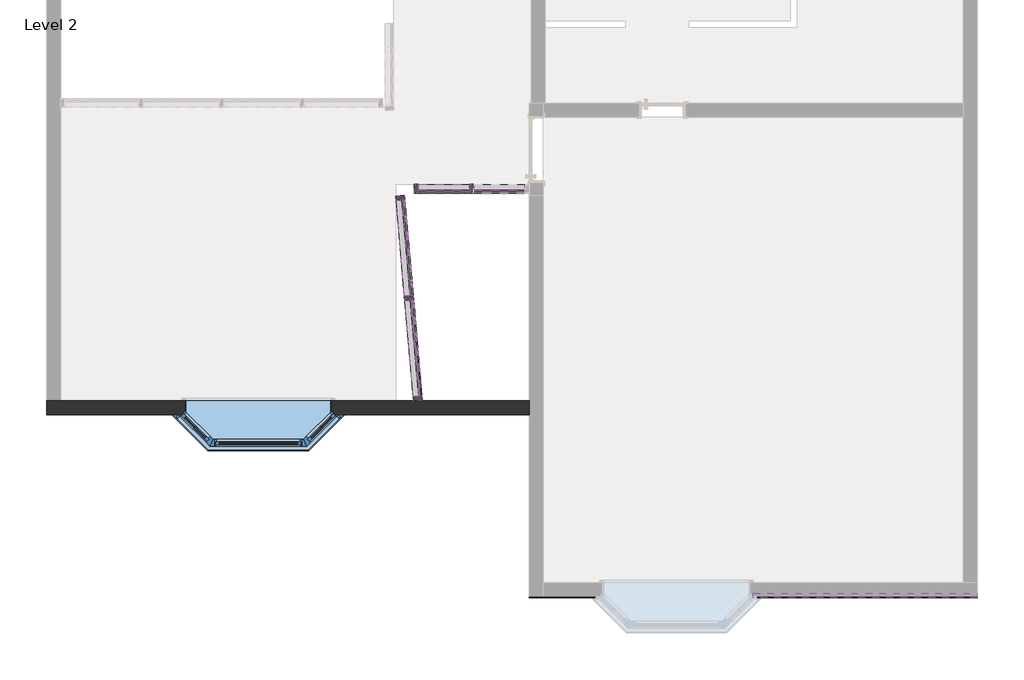
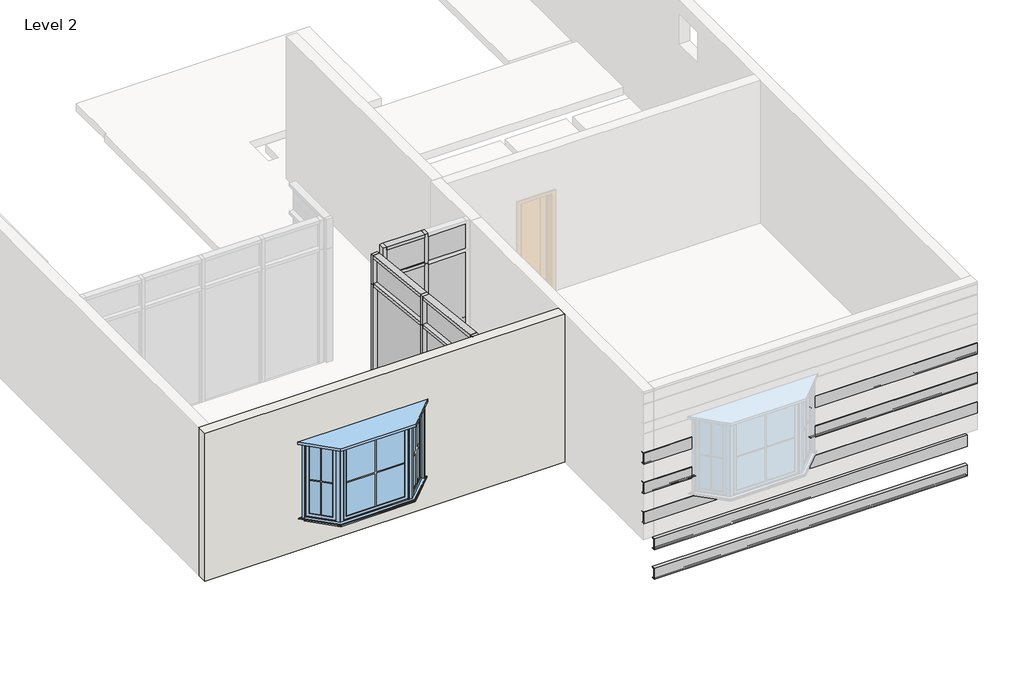
# One storey, part 2 of 5: 20 members, 8 plates, 5 proxies, 1 wall, 1 window.
"""IFC4 building model written with IfcOpenShell, lengths in millimetres."""

from ifc_helpers import new_model, si_unit, point, frame, frame_2d, origin, place, context, project, spatial, polyline, circle_curve, trimmed, segment, composite_curve, outline, extrude, faceted_brep, transform, mapped, element, save
from components import member_6e77e263, member_47bfaf8a, member_f0fea5a5, member_ee409385, member_3a0a7659, member_7b995701, member_d08ad361, member_d72f1a08, system_panel_glazed_0d615b27, system_panel_glazed_15008f27, system_panel_glazed_7a129d22, system_panel_glazed_9470322e, window_9f89e8e4

model = new_model("IFC4")

# Units and contexts
model_context = context("Model", 3, world=origin())
ifc_project = project(units=[si_unit("LENGTHUNIT", "METRE", prefix="MILLI")], contexts=[model_context])

# Site, building, storey
site = spatial("IfcSite", under=ifc_project)
building = spatial("IfcBuilding", under=site)
storey = spatial("IfcBuildingStorey", under=building, Name="Level 2", Elevation=3048.0)

# Proxies
placement = place(None, origin())
element("IfcBuildingElementProxy", 1, Name="Reveal", ObjectType="Reveal", at=placement, inside=storey, context=model_context, shape_type="SweptSolid", body=[
    extrude(outline(composite_curve([segment(polyline([(-10015.9757973, 3619.5), (-9952.7297973, 3619.5), (-9952.7297973, 3618.1203242)]), True, "CONTINUOUS"), segment(trimmed(circle_curve(frame_2d((-9957.9748973, 3618.1203242)), 5.2451), [point((-9952.7297973, 3618.1203242))], [point((-9957.1126065, 3612.9465897))], False, "CARTESIAN"), True, "CONTINUOUS"), segment(polyline([(-9957.1126065, 3612.9465897), (-9980.7332973, 3609.0098), (-9999.9711789, 3605.80348)]), True, "CONTINUOUS"), segment(trimmed(circle_curve(frame_2d((-9998.2465973, 3595.456011)), 10.4902), [point((-9999.9711789, 3605.80348))], [point((-10008.7367973, 3595.456011))], True, "CARTESIAN"), True, "CONTINUOUS"), segment(polyline([(-10008.7367973, 3595.456011), (-10008.7367973, 3414.943989)]), True, "CONTINUOUS"), segment(trimmed(circle_curve(frame_2d((-9998.2465973, 3414.943989)), 10.4902), [point((-10008.7367973, 3414.943989))], [point((-9999.9711789, 3404.59652))], True, "CARTESIAN"), True, "CONTINUOUS"), segment(polyline([(-9999.9711789, 3404.59652), (-9980.7332973, 3401.3902), (-9957.1126065, 3397.4534103)]), True, "CONTINUOUS"), segment(trimmed(circle_curve(frame_2d((-9957.9748973, 3392.2796758)), 5.2451), [point((-9957.1126065, 3397.4534103))], [point((-9952.7297973, 3392.2796758))], False, "CARTESIAN"), True, "CONTINUOUS"), segment(polyline([(-9952.7297973, 3392.2796758), (-9952.7297973, 3390.9), (-10015.9757973, 3390.9), (-10015.9757973, 3619.5)]), True, "CONTINUOUS")], self_intersect=False)), frame((-43748.9380314, 0.0, 0.0), z_axis=(1.0, 0.0, 0.0), x_axis=(0.0, 1.0, 0.0)), (0.0, 0.0, 1.0), 6502.4),
])
element("IfcBuildingElementProxy", 2, Name="Reveal", ObjectType="Reveal", at=placement, inside=storey, context=model_context, shape_type="SweptSolid", body=[
    extrude(outline(composite_curve([segment(polyline([(-10015.9757973, 4229.1), (-9952.7297973, 4229.1), (-9952.7297973, 4227.7203242)]), True, "CONTINUOUS"), segment(trimmed(circle_curve(frame_2d((-9957.9748973, 4227.7203242)), 5.2451), [point((-9952.7297973, 4227.7203242))], [point((-9957.1126065, 4222.5465897))], False, "CARTESIAN"), True, "CONTINUOUS"), segment(polyline([(-9957.1126065, 4222.5465897), (-9980.7332973, 4218.6098), (-9999.9711789, 4215.40348)]), True, "CONTINUOUS"), segment(trimmed(circle_curve(frame_2d((-9998.2465973, 4205.056011)), 10.4902), [point((-9999.9711789, 4215.40348))], [point((-10008.7367973, 4205.056011))], True, "CARTESIAN"), True, "CONTINUOUS"), segment(polyline([(-10008.7367973, 4205.056011), (-10008.7367973, 4024.543989)]), True, "CONTINUOUS"), segment(trimmed(circle_curve(frame_2d((-9998.2465973, 4024.543989)), 10.4902), [point((-10008.7367973, 4024.543989))], [point((-9999.9711789, 4014.19652))], True, "CARTESIAN"), True, "CONTINUOUS"), segment(polyline([(-9999.9711789, 4014.19652), (-9980.7332973, 4010.9902), (-9957.1126065, 4007.0534103)]), True, "CONTINUOUS"), segment(trimmed(circle_curve(frame_2d((-9957.9748973, 4001.8796758)), 5.2451), [point((-9957.1126065, 4007.0534103))], [point((-9952.7297973, 4001.8796758))], False, "CARTESIAN"), True, "CONTINUOUS"), segment(polyline([(-9952.7297973, 4001.8796758), (-9952.7297973, 4000.5), (-10015.9757973, 4000.5), (-10015.9757973, 4229.1)]), True, "CONTINUOUS")], self_intersect=False)), frame((-40499.1466227, 0.0, 0.0), z_axis=(1.0, 0.0, 0.0), x_axis=(0.0, 1.0, 0.0)), (0.0, 0.0, 1.0), 3252.6085913),
    extrude(outline(composite_curve([segment(polyline([(-10015.9757973, 4229.1), (-9952.7297973, 4229.1), (-9952.7297973, 4227.7203242)]), True, "CONTINUOUS"), segment(trimmed(circle_curve(frame_2d((-9957.9748973, 4227.7203242)), 5.2451), [point((-9952.7297973, 4227.7203242))], [point((-9957.1126065, 4222.5465897))], False, "CARTESIAN"), True, "CONTINUOUS"), segment(polyline([(-9957.1126065, 4222.5465897), (-9980.7332973, 4218.6098), (-9999.9711789, 4215.40348)]), True, "CONTINUOUS"), segment(trimmed(circle_curve(frame_2d((-9998.2465973, 4205.056011)), 10.4902), [point((-9999.9711789, 4215.40348))], [point((-10008.7367973, 4205.056011))], True, "CARTESIAN"), True, "CONTINUOUS"), segment(polyline([(-10008.7367973, 4205.056011), (-10008.7367973, 4024.543989)]), True, "CONTINUOUS"), segment(trimmed(circle_curve(frame_2d((-9998.2465973, 4024.543989)), 10.4902), [point((-10008.7367973, 4024.543989))], [point((-9999.9711789, 4014.19652))], True, "CARTESIAN"), True, "CONTINUOUS"), segment(polyline([(-9999.9711789, 4014.19652), (-9980.7332973, 4010.9902), (-9957.1126065, 4007.0534103)]), True, "CONTINUOUS"), segment(trimmed(circle_curve(frame_2d((-9957.9748973, 4001.8796758)), 5.2451), [point((-9957.1126065, 4007.0534103))], [point((-9952.7297973, 4001.8796758))], False, "CARTESIAN"), True, "CONTINUOUS"), segment(polyline([(-9952.7297973, 4001.8796758), (-9952.7297973, 4000.5), (-10015.9757973, 4000.5), (-10015.9757973, 4229.1)]), True, "CONTINUOUS")], self_intersect=False)), frame((-43748.9380314, 0.0, 0.0), z_axis=(1.0, 0.0, 0.0), x_axis=(0.0, 1.0, 0.0)), (0.0, 0.0, 1.0), 1017.4085913),
])
element("IfcBuildingElementProxy", 3, Name="Reveal", ObjectType="Reveal", at=placement, inside=storey, context=model_context, shape_type="SweptSolid", body=[
    extrude(outline(composite_curve([segment(polyline([(-10015.9757973, 4838.7), (-9952.7297973, 4838.7), (-9952.7297973, 4837.3203242)]), True, "CONTINUOUS"), segment(trimmed(circle_curve(frame_2d((-9957.9748973, 4837.3203242)), 5.2451), [point((-9952.7297973, 4837.3203242))], [point((-9957.1126065, 4832.1465897))], False, "CARTESIAN"), True, "CONTINUOUS"), segment(polyline([(-9957.1126065, 4832.1465897), (-9980.7332973, 4828.2098), (-9999.9711789, 4825.00348)]), True, "CONTINUOUS"), segment(trimmed(circle_curve(frame_2d((-9998.2465973, 4814.656011)), 10.4902), [point((-9999.9711789, 4825.00348))], [point((-10008.7367973, 4814.656011))], True, "CARTESIAN"), True, "CONTINUOUS"), segment(polyline([(-10008.7367973, 4814.656011), (-10008.7367973, 4634.143989)]), True, "CONTINUOUS"), segment(trimmed(circle_curve(frame_2d((-9998.2465973, 4634.143989)), 10.4902), [point((-10008.7367973, 4634.143989))], [point((-9999.9711789, 4623.79652))], True, "CARTESIAN"), True, "CONTINUOUS"), segment(polyline([(-9999.9711789, 4623.79652), (-9980.7332973, 4620.5902), (-9957.1126065, 4616.6534103)]), True, "CONTINUOUS"), segment(trimmed(circle_curve(frame_2d((-9957.9748973, 4611.4796758)), 5.2451), [point((-9957.1126065, 4616.6534103))], [point((-9952.7297973, 4611.4796758))], False, "CARTESIAN"), True, "CONTINUOUS"), segment(polyline([(-9952.7297973, 4611.4796758), (-9952.7297973, 4610.1), (-10015.9757973, 4610.1), (-10015.9757973, 4838.7)]), True, "CONTINUOUS")], self_intersect=False)), frame((-40499.1466227, 0.0, 0.0), z_axis=(1.0, 0.0, 0.0), x_axis=(0.0, 1.0, 0.0)), (0.0, 0.0, 1.0), 3252.6085913),
    extrude(outline(composite_curve([segment(polyline([(-10015.9757973, 4838.7), (-9952.7297973, 4838.7), (-9952.7297973, 4837.3203242)]), True, "CONTINUOUS"), segment(trimmed(circle_curve(frame_2d((-9957.9748973, 4837.3203242)), 5.2451), [point((-9952.7297973, 4837.3203242))], [point((-9957.1126065, 4832.1465897))], False, "CARTESIAN"), True, "CONTINUOUS"), segment(polyline([(-9957.1126065, 4832.1465897), (-9980.7332973, 4828.2098), (-9999.9711789, 4825.00348)]), True, "CONTINUOUS"), segment(trimmed(circle_curve(frame_2d((-9998.2465973, 4814.656011)), 10.4902), [point((-9999.9711789, 4825.00348))], [point((-10008.7367973, 4814.656011))], True, "CARTESIAN"), True, "CONTINUOUS"), segment(polyline([(-10008.7367973, 4814.656011), (-10008.7367973, 4634.143989)]), True, "CONTINUOUS"), segment(trimmed(circle_curve(frame_2d((-9998.2465973, 4634.143989)), 10.4902), [point((-10008.7367973, 4634.143989))], [point((-9999.9711789, 4623.79652))], True, "CARTESIAN"), True, "CONTINUOUS"), segment(polyline([(-9999.9711789, 4623.79652), (-9980.7332973, 4620.5902), (-9957.1126065, 4616.6534103)]), True, "CONTINUOUS"), segment(trimmed(circle_curve(frame_2d((-9957.9748973, 4611.4796758)), 5.2451), [point((-9957.1126065, 4616.6534103))], [point((-9952.7297973, 4611.4796758))], False, "CARTESIAN"), True, "CONTINUOUS"), segment(polyline([(-9952.7297973, 4611.4796758), (-9952.7297973, 4610.1), (-10015.9757973, 4610.1), (-10015.9757973, 4838.7)]), True, "CONTINUOUS")], self_intersect=False)), frame((-43748.9380314, 0.0, 0.0), z_axis=(1.0, 0.0, 0.0), x_axis=(0.0, 1.0, 0.0)), (0.0, 0.0, 1.0), 1017.4085913),
])
element("IfcBuildingElementProxy", 4, Name="Reveal", ObjectType="Reveal", at=placement, inside=storey, context=model_context, shape_type="SweptSolid", body=[
    extrude(outline(composite_curve([segment(polyline([(-10015.9757973, 2400.3), (-9952.7297973, 2400.3), (-9952.7297973, 2398.9203242)]), True, "CONTINUOUS"), segment(trimmed(circle_curve(frame_2d((-9957.9748973, 2398.9203242)), 5.2451), [point((-9952.7297973, 2398.9203242))], [point((-9957.1126065, 2393.7465897))], False, "CARTESIAN"), True, "CONTINUOUS"), segment(polyline([(-9957.1126065, 2393.7465897), (-9980.7332973, 2389.8098), (-9999.9711789, 2386.60348)]), True, "CONTINUOUS"), segment(trimmed(circle_curve(frame_2d((-9998.2465973, 2376.256011)), 10.4902), [point((-9999.9711789, 2386.60348))], [point((-10008.7367973, 2376.256011))], True, "CARTESIAN"), True, "CONTINUOUS"), segment(polyline([(-10008.7367973, 2376.256011), (-10008.7367973, 2195.743989)]), True, "CONTINUOUS"), segment(trimmed(circle_curve(frame_2d((-9998.2465973, 2195.743989)), 10.4902), [point((-10008.7367973, 2195.743989))], [point((-9999.9711789, 2185.39652))], True, "CARTESIAN"), True, "CONTINUOUS"), segment(polyline([(-9999.9711789, 2185.39652), (-9980.7332973, 2182.1902), (-9957.1126065, 2178.2534103)]), True, "CONTINUOUS"), segment(trimmed(circle_curve(frame_2d((-9957.9748973, 2173.0796758)), 5.2451), [point((-9957.1126065, 2178.2534103))], [point((-9952.7297973, 2173.0796758))], False, "CARTESIAN"), True, "CONTINUOUS"), segment(polyline([(-9952.7297973, 2173.0796758), (-9952.7297973, 2171.7), (-10015.9757973, 2171.7), (-10015.9757973, 2400.3)]), True, "CONTINUOUS")], self_intersect=False)), frame((-43545.7380314, 0.0, 0.0), z_axis=(1.0, 0.0, 0.0), x_axis=(0.0, 1.0, 0.0)), (0.0, 0.0, 1.0), 6096.0),
])
element("IfcBuildingElementProxy", 5, Name="Reveal", ObjectType="Reveal", at=placement, inside=storey, context=model_context, shape_type="SweptSolid", body=[
    extrude(outline(composite_curve([segment(polyline([(-10015.9757973, 3009.9), (-9952.7297973, 3009.9), (-9952.7297973, 3008.5203242)]), True, "CONTINUOUS"), segment(trimmed(circle_curve(frame_2d((-9957.9748973, 3008.5203242)), 5.2451), [point((-9952.7297973, 3008.5203242))], [point((-9957.1126065, 3003.3465897))], False, "CARTESIAN"), True, "CONTINUOUS"), segment(polyline([(-9957.1126065, 3003.3465897), (-9980.7332973, 2999.4098), (-9999.9711789, 2996.20348)]), True, "CONTINUOUS"), segment(trimmed(circle_curve(frame_2d((-9998.2465973, 2985.856011)), 10.4902), [point((-9999.9711789, 2996.20348))], [point((-10008.7367973, 2985.856011))], True, "CARTESIAN"), True, "CONTINUOUS"), segment(polyline([(-10008.7367973, 2985.856011), (-10008.7367973, 2805.343989)]), True, "CONTINUOUS"), segment(trimmed(circle_curve(frame_2d((-9998.2465973, 2805.343989)), 10.4902), [point((-10008.7367973, 2805.343989))], [point((-9999.9711789, 2794.99652))], True, "CARTESIAN"), True, "CONTINUOUS"), segment(polyline([(-9999.9711789, 2794.99652), (-9980.7332973, 2791.7902), (-9957.1126065, 2787.8534103)]), True, "CONTINUOUS"), segment(trimmed(circle_curve(frame_2d((-9957.9748973, 2782.6796758)), 5.2451), [point((-9957.1126065, 2787.8534103))], [point((-9952.7297973, 2782.6796758))], False, "CARTESIAN"), True, "CONTINUOUS"), segment(polyline([(-9952.7297973, 2782.6796758), (-9952.7297973, 2781.3), (-10015.9757973, 2781.3), (-10015.9757973, 3009.9)]), True, "CONTINUOUS")], self_intersect=False)), frame((-43545.7380314, 0.0, 0.0), z_axis=(1.0, 0.0, 0.0), x_axis=(0.0, 1.0, 0.0)), (0.0, 0.0, 1.0), 6096.0),
])

# Members
member_shape = member_6e77e263(model_context)
element("IfcMember", 6, ObjectType="Rectangular Mullion : 2.5\" x 5\" rectangular", at=placement, inside=storey, context=model_context, shape_type="MappedRepresentation", body=[
    mapped(member_shape, transform((-44587.1380314, -4081.0930974, 5486.4), x_axis=(1.0, 0.0, 0.0), y_axis=(0.0, -1.0, 0.0), z_axis=(0.0, 0.0, -1.0))),
])
element("IfcMember", 7, ObjectType="Rectangular Mullion : 2.5\" x 5\" rectangular", at=placement, inside=storey, context=model_context, shape_type="MappedRepresentation", body=[
    mapped(member_shape, transform((-45498.4599609, -5669.4922473, 5486.4), x_axis=(-0.08715574274765692, 0.9961946980917457, 0.0), y_axis=(0.9961946980917457, 0.08715574274765692, 0.0), z_axis=(0.0, 0.0, -1.0))),
])
member_2_shape = member_47bfaf8a(model_context)
element("IfcMember", 8, ObjectType="Rectangular Mullion : 2.5\" x 5\" rectangular", at=placement, inside=storey, context=model_context, shape_type="MappedRepresentation", body=[
    mapped(member_2_shape, transform((-45425.3380314, -4081.0930974, 6096.0), x_axis=(-1.0, 0.0, 0.0), y_axis=(0.0, -1.0, 0.0), z_axis=(0.0, 0.0, 1.0))),
])
element("IfcMember", 9, ObjectType="Rectangular Mullion : 2.5\" x 5\" rectangular", at=placement, inside=storey, context=model_context, shape_type="MappedRepresentation", body=[
    mapped(member_2_shape, transform((-45368.3818903, -7156.2913973, 6096.0), x_axis=(0.08715574274765692, -0.9961946980917457, 0.0), y_axis=(0.9961946980917457, 0.08715574274765692, 0.0), z_axis=(0.0, 0.0, 1.0))),
])
element("IfcMember", 10, ObjectType="Rectangular Mullion : 2.5\" x 5\" rectangular", at=placement, inside=storey, context=model_context, shape_type="MappedRepresentation", body=[
    mapped(member_2_shape, transform((-45628.5380314, -4182.6930974, 5486.4), x_axis=(-0.08715574274765692, 0.9961946980917457, 0.0), y_axis=(0.9961946980917457, 0.08715574274765692, 0.0), z_axis=(0.0, 0.0, -1.0))),
])
member_3_shape = member_f0fea5a5(model_context)
element("IfcMember", 11, ObjectType="Rectangular Mullion : 2.5\" x 5\" rectangular", at=placement, inside=storey, context=model_context, shape_type="MappedRepresentation", body=[
    mapped(member_3_shape, transform((-44587.1380314, -4081.0930974, 3048.0), x_axis=(1.0, 0.0, 0.0), y_axis=(0.0, -1.0, 0.0), z_axis=(0.0, 0.0, -1.0))),
])
element("IfcMember", 12, ObjectType="Rectangular Mullion : 2.5\" x 5\" rectangular", at=placement, inside=storey, context=model_context, shape_type="MappedRepresentation", body=[
    mapped(member_3_shape, transform((-45498.4599609, -5669.4922473, 3048.0), x_axis=(-0.08715574274765692, 0.9961946980917457, 0.0), y_axis=(0.9961946980917457, 0.08715574274765692, 0.0), z_axis=(0.0, 0.0, -1.0))),
])
member_4_shape = member_ee409385(model_context)
element("IfcMember", 13, ObjectType="Rectangular Mullion : 2.5\" x 5\" rectangular", at=placement, inside=storey, context=model_context, shape_type="MappedRepresentation", body=[
    mapped(member_4_shape, transform((-45628.5380314, -4182.6930974, 3048.0), x_axis=(-0.08715574274765692, 0.9961946980917457, 0.0), y_axis=(0.9961946980917457, 0.08715574274765692, 0.0), z_axis=(0.0, 0.0, -1.0))),
])
element("IfcMember", 14, ObjectType="Rectangular Mullion : 2.5\" x 5\" rectangular", at=placement, inside=storey, context=model_context, shape_type="MappedRepresentation", body=[
    mapped(member_4_shape, transform((-45425.3380314, -4081.0930974, 5486.4), x_axis=(-1.0, 0.0, 0.0), y_axis=(0.0, -1.0, 0.0), z_axis=(0.0, 0.0, 1.0))),
])
element("IfcMember", 15, ObjectType="Rectangular Mullion : 2.5\" x 5\" rectangular", at=placement, inside=storey, context=model_context, shape_type="MappedRepresentation", body=[
    mapped(member_4_shape, transform((-45368.3818903, -7156.2913973, 5486.4), x_axis=(0.08715574274765692, -0.9961946980917457, 0.0), y_axis=(0.9961946980917457, 0.08715574274765692, 0.0), z_axis=(0.0, 0.0, 1.0))),
])
member_5_shape = member_3a0a7659(model_context)
element("IfcMember", 16, ObjectType="Rectangular Mullion : 2.5\" x 5\" rectangular", at=placement, inside=storey, context=model_context, shape_type="MappedRepresentation", body=[
    mapped(member_5_shape, transform((-44618.8880314, -4081.0930974, 6096.0), x_axis=(0.0, 0.0, 1.0), y_axis=(0.0, -1.0, 0.0), z_axis=(1.0, 0.0, 0.0))),
])
element("IfcMember", 17, ObjectType="Rectangular Mullion : 2.5\" x 5\" rectangular", at=placement, inside=storey, context=model_context, shape_type="MappedRepresentation", body=[
    mapped(member_5_shape, transform((-45361.8380314, -4081.0930974, 3048.0), x_axis=(0.0, 0.0, -1.0), y_axis=(0.0, -1.0, 0.0), z_axis=(-1.0, 0.0, 0.0))),
])
element("IfcMember", 18, ObjectType="Rectangular Mullion : 2.5\" x 5\" rectangular", at=placement, inside=storey, context=model_context, shape_type="MappedRepresentation", body=[
    mapped(member_5_shape, transform((-44555.3880314, -4081.0930974, 3048.0), x_axis=(0.0, 0.0, -1.0), y_axis=(0.0, -1.0, 0.0), z_axis=(-1.0, 0.0, 0.0))),
])
member_6_shape = member_7b995701(model_context)
element("IfcMember", 19, ObjectType="Rectangular Mullion : 2.5\" x 5\" rectangular", at=placement, inside=storey, context=model_context, shape_type="MappedRepresentation", body=[
    mapped(member_6_shape, transform((-44618.8880314, -4081.0930974, 5486.4), x_axis=(0.0, 0.0, 1.0), y_axis=(0.0, -1.0, 0.0), z_axis=(1.0, 0.0, 0.0))),
])
member_7_shape = member_d08ad361(model_context)
element("IfcMember", 20, ObjectType="Rectangular Mullion : 2.5\" x 5\" rectangular", at=placement, inside=storey, context=model_context, shape_type="MappedRepresentation", body=[
    mapped(member_7_shape, transform((-45623.0036418, -4245.9514607, 6096.0), x_axis=(0.0, 0.0, 1.0), y_axis=(0.9961946980917455, 0.08715574274765832, 0.0), z_axis=(-0.0871557427476583, 0.9961946980917454, 0.0))),
])
element("IfcMember", 21, ObjectType="Rectangular Mullion : 2.5\" x 5\" rectangular", at=placement, inside=storey, context=model_context, shape_type="MappedRepresentation", body=[
    mapped(member_7_shape, transform((-45495.692766, -5701.121429, 6096.0), x_axis=(0.0, 0.0, 1.0), y_axis=(0.9961946980917454, 0.08715574274765911, 0.0), z_axis=(-0.08715574274765911, 0.9961946980917454, 0.0))),
])
element("IfcMember", 22, ObjectType="Rectangular Mullion : 2.5\" x 5\" rectangular", at=placement, inside=storey, context=model_context, shape_type="MappedRepresentation", body=[
    mapped(member_7_shape, transform((-45373.91628, -7093.0330339, 3048.0), x_axis=(0.0, 0.0, -1.0), y_axis=(0.9961946980917454, 0.08715574274765911, 0.0), z_axis=(0.08715574274765911, -0.9961946980917454, 0.0))),
])
element("IfcMember", 23, ObjectType="Rectangular Mullion : 2.5\" x 5\" rectangular", at=placement, inside=storey, context=model_context, shape_type="MappedRepresentation", body=[
    mapped(member_7_shape, transform((-45501.2271557, -5637.8630656, 3048.0), x_axis=(0.0, 0.0, -1.0), y_axis=(0.9961946980917454, 0.08715574274765905, 0.0), z_axis=(0.08715574274765905, -0.9961946980917454, 0.0))),
])
member_8_shape = member_d72f1a08(model_context)
element("IfcMember", 24, ObjectType="Rectangular Mullion : 2.5\" x 5\" rectangular", at=placement, inside=storey, context=model_context, shape_type="MappedRepresentation", body=[
    mapped(member_8_shape, transform((-45623.0036418, -4245.9514607, 5486.4), x_axis=(0.0, 0.0, 1.0), y_axis=(0.9961946980917455, 0.08715574274765832, 0.0), z_axis=(-0.0871557427476583, 0.9961946980917454, 0.0))),
])
element("IfcMember", 25, ObjectType="Rectangular Mullion : 2.5\" x 5\" rectangular", at=placement, inside=storey, context=model_context, shape_type="MappedRepresentation", body=[
    mapped(member_8_shape, transform((-45495.692766, -5701.121429, 5486.4), x_axis=(0.0, 0.0, 1.0), y_axis=(0.9961946980917454, 0.08715574274765911, 0.0), z_axis=(-0.08715574274765911, 0.9961946980917454, 0.0))),
])

# Plates
system_panel_glazed_shape = system_panel_glazed_0d615b27(model_context)
element("IfcPlate", 26, ObjectType="System Panel : Glazed", at=placement, inside=storey, context=model_context, shape_type="MappedRepresentation", body=[
    mapped(system_panel_glazed_shape, transform((-44990.3630314, -4081.0930974, 3111.5), x_axis=(1.0, 0.0, 0.0), y_axis=(0.0, 1.0, 0.0), z_axis=(0.0, 0.0, 1.0))),
])
element("IfcPlate", 27, ObjectType="System Panel : Glazed", at=placement, inside=storey, context=model_context, shape_type="MappedRepresentation", body=[
    mapped(system_panel_glazed_shape, transform((-44183.9130314, -4081.0930974, 3111.5), x_axis=(1.0, 0.0, 0.0), y_axis=(0.0, 1.0, 0.0), z_axis=(0.0, 0.0, 1.0))),
])
system_panel_glazed_2_shape = system_panel_glazed_15008f27(model_context)
element("IfcPlate", 28, ObjectType="System Panel : Glazed", at=placement, inside=storey, context=model_context, shape_type="MappedRepresentation", body=[
    mapped(system_panel_glazed_2_shape, transform((-44990.3630314, -4081.0930974, 5518.15), x_axis=(1.0, 0.0, 0.0), y_axis=(0.0, 1.0, 0.0), z_axis=(0.0, 0.0, 1.0))),
])
element("IfcPlate", 29, ObjectType="System Panel : Glazed", at=placement, inside=storey, context=model_context, shape_type="MappedRepresentation", body=[
    mapped(system_panel_glazed_2_shape, transform((-44183.9130314, -4081.0930974, 5518.15), x_axis=(1.0, 0.0, 0.0), y_axis=(0.0, 1.0, 0.0), z_axis=(0.0, 0.0, 1.0))),
])
system_panel_glazed_3_shape = system_panel_glazed_7a129d22(model_context)
element("IfcPlate", 30, ObjectType="System Panel : Glazed", at=placement, inside=storey, context=model_context, shape_type="MappedRepresentation", body=[
    mapped(system_panel_glazed_3_shape, transform((-45434.804523, -6397.0772315, 3111.5), x_axis=(-0.08715574274765692, 0.9961946980917457, 0.0), y_axis=(-0.9961946980917457, -0.08715574274765692, 0.0), z_axis=(0.0, 0.0, 1.0))),
])
element("IfcPlate", 31, ObjectType="System Panel : Glazed", at=placement, inside=storey, context=model_context, shape_type="MappedRepresentation", body=[
    mapped(system_panel_glazed_3_shape, transform((-45562.1153987, -4941.9072632, 3111.5), x_axis=(-0.08715574274765692, 0.9961946980917457, 0.0), y_axis=(-0.9961946980917457, -0.08715574274765692, 0.0), z_axis=(0.0, 0.0, 1.0))),
])
system_panel_glazed_4_shape = system_panel_glazed_9470322e(model_context)
element("IfcPlate", 32, ObjectType="System Panel : Glazed", at=placement, inside=storey, context=model_context, shape_type="MappedRepresentation", body=[
    mapped(system_panel_glazed_4_shape, transform((-45434.804523, -6397.0772315, 5518.15), x_axis=(-0.08715574274765692, 0.9961946980917457, 0.0), y_axis=(-0.9961946980917457, -0.08715574274765692, 0.0), z_axis=(0.0, 0.0, 1.0))),
])
element("IfcPlate", 33, ObjectType="System Panel : Glazed", at=placement, inside=storey, context=model_context, shape_type="MappedRepresentation", body=[
    mapped(system_panel_glazed_4_shape, transform((-45562.1153987, -4941.9072632, 5518.15), x_axis=(-0.08715574274765692, 0.9961946980917457, 0.0), y_axis=(-0.9961946980917457, -0.08715574274765692, 0.0), z_axis=(0.0, 0.0, 1.0))),
])

# Wall
element("IfcWall", 34, ObjectType="OUTER WALL 8\"", at=placement, inside=storey, context=model_context, shape_type="Brep", body=[
    faceted_brep([(-50759.3380314, -7359.4913973, 3048.0), (-43748.9380314, -7359.4913973, 3048.0), (-43748.9380314, -7359.4913973, 6096.0), (-50759.3380314, -7359.4913973, 6096.0), (-48802.1294401, -7359.4913973, 5232.4), (-46569.7466227, -7359.4913973, 5232.4), (-46569.7466227, -7359.4913973, 3657.6), (-48802.1294401, -7359.4913973, 3657.6), (-50759.3380314, -7156.2913973, 3048.0), (-50759.3380314, -7156.2913973, 6096.0), (-50556.1380314, -7156.2913973, 6096.0), (-43748.9380314, -7156.2913973, 6096.0), (-43748.9380314, -7156.2913973, 3048.0), (-50556.1380314, -7156.2913973, 3048.0), (-46619.1380314, -7156.2913973, 5232.4), (-48752.7380314, -7156.2913973, 5232.4), (-48752.7380314, -7156.2913973, 3657.6), (-46619.1380314, -7156.2913973, 3657.6), (-46619.1380314, -7310.0999886, 5232.4), (-48752.7380314, -7310.0999886, 5232.4), (-46619.1380314, -7310.0999886, 3657.6), (-48752.7380314, -7310.0999886, 3657.6)], [[[0, 1, 2, 3], [4, 5, 6, 7]], [[8, 9, 10, 11, 12, 13], [14, 15, 16, 17]], [[1, 0, 8, 13, 12]], [[3, 2, 11, 10, 9]], [[0, 3, 9, 8]], [[18, 5, 4, 19, 15, 14]], [[20, 17, 16, 21, 7, 6]], [[18, 14, 17, 20]], [[15, 19, 21, 16]], [[19, 4, 7, 21]], [[5, 18, 20, 6]], [[2, 1, 12, 11]]]),
])

# Window
window_shape = window_9f89e8e4(model_context)
element("IfcWindow", 35, ObjectType="Window-Bay-Casement-45_Degree_Angle : 84\" x 60\" x 18\"", at=placement, inside=storey, context=model_context, shape_type="MappedRepresentation", body=[
    mapped(window_shape, transform((-47685.9380314, -7257.8913973, 3048.0), x_axis=(-1.0, 0.0, 0.0), y_axis=(0.0, -1.0, 0.0), z_axis=(0.0, 0.0, 1.0))),
])

save(model, "model.ifc")

# Revit data of these elements
# Type "Rectangular Mullion : 2.5\" x 5\" rectangular"
#   built-in parameter 1007304 = 0.416667 (stored number, unit not read)
#   built-in parameter 1007301 = 0.104167 (stored number, unit not read)
#   built-in parameter 1007300 = 0.104167 (stored number, unit not read)
# Type "System Panel : Glazed"
#   Construction Type Id = "GSP4R"
#   Analytic Construction = "1/8 in Pilkington single glazing"
#   Visual Light Transmittance = 0.9
#   Solar Heat Gain Coefficient = 0.86
#   Heat Transfer Coefficient (U) = 1.18115 BTU/(h·ft²·°F)
#   Define Thermal Properties by = 1
# Type "OUTER WALL 8\""
#   Assembly Code = "B2010"
#   Layers, outside or top first: 0' - 8" "BEIGE COLOUR" (function 1)
# Type "Window-Bay-Casement-45_Degree_Angle : 84\" x 60\" x 18\""
#   Type Mark = "18"
#   Fire Rating = "0.5h"
#   Assembly Code = "B2020100"
#   Analytic Construction = "Double glazing - domestic"
#   Width of Middle Sash = 4' - 2.38909"
#   Width = 7' - 0"
#   Visual Light Transmittance = 0.81
#   Thermal Resistance (R) = 1.8146 (h·ft²·°F)/BTU
#   Solar Heat Gain Coefficient = 0.76
#   Rough Width = 7' - 0 1/2"
#   Rough Height = 5' - 0 1/2"
#   Length 4 = 0' - 1.13909"
#   Length 3 = 0' - 0.51777"
#   Length 2 = 4' - 7.42462"
#   Length 1 = 1' - 2.80546"
#   Wall Thickness [instance default] = 0' - 6"
#   Trim Width = 7' - 5.03553"
#   Trim Height = 5' - 0"
#   Height 1 = 5' - 2"
#   Height = 5' - 0"
#   Heat Transfer Coefficient (U) = 0.5511 BTU/(h·ft²·°F)
#   Depth = 1' - 6"
#   Default Sill Height = 2' - 0"
#   Angle 1 = 22.50°
#   Angle = 45.00°
#   Center Muntin Visibility = yes
#   Side Muntin Visibility = yes
#   Interior Trim Visibility [instance default] = yes
#   Exterior Trim Visibility [instance default] = yes
#   Center Muntin Pattern = Muntin Pattern_2x2 : Muntin Pattern_2x2
#   Side Muntin Pattern = Muntin Pattern_2x2 : Muntin Pattern_2x2
#   Interior Trim Material = Wood - Stained
#   Exterior Trim Material = Clad - White
#   Exterior Trim = element 406231
#   Interior Trim = Trim-Window-Interior-Flat : Picture Frame
#   Interior Frame Material = Wood - Stained
#   Glass Panel Material = Glass
#   Exterior Frame Material = Clad - White
#   Wall Closure = (empty or 0)
# Elements 6, 7, 8, 9, 10, 11, 12, 13, 14, 15, 16, 17, 18, 19, 20, 21, 22, 23, 24, 25 (IfcMember, "Rectangular Mullion : 2.5\" x 5\" rectangular")
#   Phase Created = New Construction
#   Materials on its faces: "Aluminum"
# Elements 26, 27, 28, 29, 30, 31, 32, 33 (IfcPlate, "System Panel : Glazed")
#   Phase Created = New Construction
#   Materials on its faces: "glass panel 223"
# Element 34 (IfcWall, "OUTER WALL 8\"")
#   Top Offset = 0' - 0"
#   Base Offset = 0' - 0"
#   wall height = 10' - 0"
#   Phase Created = New Construction
#   Base Constraint = Level 2
#   Top Constraint = Level 3
#   Materials on its faces: "BEIGE COLOUR"
# Element 35 (IfcWindow, "Window-Bay-Casement-45_Degree_Angle : 84\" x 60\" x 18\"")
#   Mark = "13"
#   Interior Trim Visibility = yes
#   Exterior Trim Visibility = yes
#   Phase Created = New Construction
#   Materials on its faces: "Wood - Stained", "Clad - White", "Glass"
# Materials
#   "BEIGE COLOUR": class "Generic", colour RGB 120 120 120, transparency 0, Cost = 0
#   "Wood - Stained": class "Wood", colour RGB 224 178 126, transparency 0, Cost = 0
#   "Clad - White": class "Wood", colour RGB 242 242 238, transparency 0, Cost = 0
#   "Glass": class "Glass", colour RGB 0 128 192, transparency 0.75, Description = "Soda Lime Glass", Cost = 0
#   "Aluminum": class "Metal", colour RGB 247 247 247, transparency 0, Description = "Aluminum 6061", Cost = 0
#   "glass panel 223": class "Generic", colour RGB 120 120 120, transparency 0, Cost = 0
